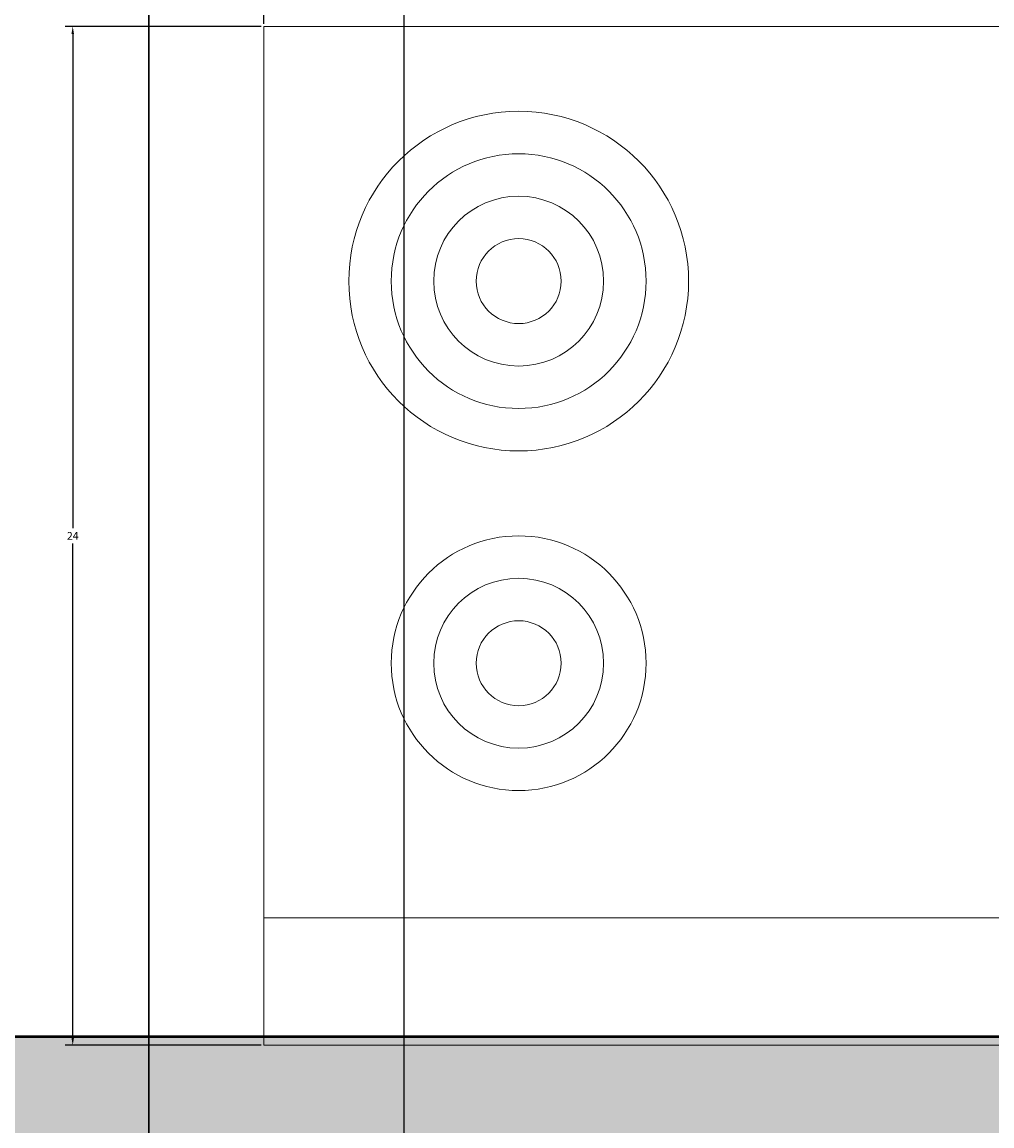
# Model space of a CAD drawing. Units: inches. Extents: x 2307 to 2544, y 2171 to 2540.
# Tile 30 of 52: x 2453 to 2476, y 2317 to 2343. Entities that reach past the tile are written whole.
import ezdxf

# ---------------------------------------------------------------- set-up
doc = ezdxf.new("R2010")
doc.units = ezdxf.units.IN
for name, color, linetype, lineweight in [('A-ANNO-DIMS', 2, 'Continuous', 18), ('A-EQPM', 8, 'Continuous', 18), ('A-WALL', 7, 'Continuous', 50)]:
    doc.layers.add(name, color=color, linetype=linetype, lineweight=lineweight)
doc.layers.add('A-WALL-PATT', color=18, linetype='Continuous', lineweight=13, true_color=0x000000)
doc.styles.get("Standard").update_dxf_attribs({"font": 'arial.ttf'})
doc.dimstyles.get("Standard").update_dxf_attribs({"dimtxt": 0.18, "dimasz": 0.18, "dimexe": 0.18, "dimexo": 0.0625, "dimgap": 0.09, "dimtad": 0, "dimtih": 1, "dimtoh": 1, "dimdec": 4, "dimzin": 0, "dimdsep": 46, "dimtxsty": 'Standard', "dimcen": 0.09, "dimadec": 0, "dimazin": 0, "dimtfac": 1, "dimtdec": 4, "dimtofl": 0, "dimtmove": 0, "dimatfit": 3, "dimfxl": 1, "dimtolj": 1, "dimtzin": 0, "dimarcsym": 0})

# ---------------------------------------------------------------- blocks, each defined once
blk = doc.blocks.new('Range-Oven - 30 in top')
blk.add_line((0, -3), (30, -3))
blk.add_lwpolyline([(0, -24), (0, 0), (30, 0), (30, -24)], close=True)
for centre, radius in [((6, -9), 4), ((6, -9), 3), ((24, -9), 3), ((6, -9), 2), ((24, -9), 2), ((6, -9), 1), ((24, -9), 1), ((24, -18), 4), ((6, -18), 3), ((24, -18), 3), ((6, -18), 2), ((24, -18), 2), ((6, -18), 1), ((24, -18), 1)]:
    blk.add_circle(centre, radius)
blk = doc.blocks.new('*D30')
at = {"layer": 'A-ANNO-DIMS', "color": 0, "lineweight": -2, "transparency": 16777216}
for p, q in [((2458.401, 2343.369), (2458.401, 2347.987)), ((2458.581, 2347.807), (2472.705, 2347.807)), ((2488.221, 2347.807), (2474.097, 2347.807)), ((2488.401, 2343.369), (2488.401, 2347.987))]:
    blk.add_line(p, q, dxfattribs=at)
at = {"layer": 'A-ANNO-DIMS', "color": 0, "transparency": 16777216}
for points in [[(2458.581, 2347.837), (2458.581, 2347.777), (2458.401, 2347.807)], [(2488.221, 2347.837), (2488.221, 2347.777), (2488.401, 2347.807)]]:
    blk.add_solid(points, dxfattribs=at)
at = {"layer": 'Defpoints', "color": 0, "transparency": 16777216}
for p in [(2458.401, 2347.807), (2458.401, 2343.307), (2488.401, 2343.307)]:
    blk.add_point(p, dxfattribs=at)
at = {"layer": 'A-ANNO-DIMS', "color": 0, "transparency": 16777216, "insert": (2473.401, 2347.807), "char_height": 0.18, "attachment_point": 5}
blk.add_mtext('\\A1;RANGE 30', dxfattribs=at)
blk = doc.blocks.new('*D31')
at = {"layer": 'A-ANNO-DIMS', "color": 0, "lineweight": -2, "transparency": 16777216}
for p, q in [((2458.339, 2343.307), (2453.721, 2343.307)), ((2453.901, 2343.127), (2453.901, 2331.487)), ((2453.901, 2319.487), (2453.901, 2331.126)), ((2458.339, 2319.307), (2453.721, 2319.307))]:
    blk.add_line(p, q, dxfattribs=at)
at = {"layer": 'A-ANNO-DIMS', "color": 0, "transparency": 16777216}
for points in [[(2453.871, 2343.127), (2453.931, 2343.127), (2453.901, 2343.307)], [(2453.871, 2319.487), (2453.931, 2319.487), (2453.901, 2319.307)]]:
    blk.add_solid(points, dxfattribs=at)
at = {"layer": 'Defpoints', "color": 0, "transparency": 16777216}
for p in [(2458.401, 2343.307), (2453.901, 2319.307), (2458.401, 2319.307)]:
    blk.add_point(p, dxfattribs=at)
at = {"layer": 'A-ANNO-DIMS', "color": 0, "transparency": 16777216, "insert": (2453.901, 2331.307), "char_height": 0.18, "attachment_point": 5}
blk.add_mtext('\\A1;24', dxfattribs=at)
blk = doc.blocks.new('*D53')
at = {"layer": 'A-ANNO-DIMS', "color": 0, "lineweight": -2, "transparency": 16777216}
for p, q in [((2455.696, 2439.447), (2455.696, 2171.18)), ((2461.696, 2439.447), (2461.696, 2171.18)), ((2455.876, 2171.36), (2458.546, 2171.36)), ((2461.516, 2171.36), (2458.845, 2171.36))]:
    blk.add_line(p, q, dxfattribs=at)
at = {"layer": 'A-ANNO-DIMS', "color": 0, "transparency": 16777216}
for points in [[(2455.876, 2171.39), (2455.876, 2171.33), (2455.696, 2171.36)], [(2461.516, 2171.39), (2461.516, 2171.33), (2461.696, 2171.36)]]:
    blk.add_solid(points, dxfattribs=at)
at = {"layer": 'Defpoints', "color": 0, "transparency": 16777216}
for p in [(2455.696, 2439.51), (2461.696, 2439.51), (2461.696, 2171.36)]:
    blk.add_point(p, dxfattribs=at)
at = {"layer": 'A-ANNO-DIMS', "color": 0, "transparency": 16777216, "insert": (2458.696, 2171.36), "char_height": 0.18, "attachment_point": 5}
blk.add_mtext('\\A1;6', dxfattribs=at)
blk = doc.blocks.new('*D54')
at = {"layer": 'A-ANNO-DIMS', "color": 0, "lineweight": -2, "transparency": 16777216}
for p, q in [((2461.696, 2435.447), (2461.696, 2171.18)), ((2491.696, 2435.447), (2491.696, 2171.18)), ((2461.876, 2171.36), (2476.477, 2171.36)), ((2491.516, 2171.36), (2476.914, 2171.36))]:
    blk.add_line(p, q, dxfattribs=at)
at = {"layer": 'A-ANNO-DIMS', "color": 0, "transparency": 16777216}
for points in [[(2461.876, 2171.39), (2461.876, 2171.33), (2461.696, 2171.36)], [(2491.516, 2171.39), (2491.516, 2171.33), (2491.696, 2171.36)]]:
    blk.add_solid(points, dxfattribs=at)
at = {"layer": 'Defpoints', "color": 0, "transparency": 16777216}
for p in [(2461.696, 2435.51), (2491.696, 2435.51), (2491.696, 2171.36)]:
    blk.add_point(p, dxfattribs=at)
at = {"layer": 'A-ANNO-DIMS', "color": 0, "transparency": 16777216, "insert": (2476.696, 2171.36), "char_height": 0.18, "attachment_point": 5}
blk.add_mtext('\\A1;30', dxfattribs=at)
blk = doc.blocks.new('*D59')
at = {"layer": 'A-ANNO-DIMS', "color": 0, "lineweight": -2, "transparency": 16777216}
for p, q in [((2455.696, 2315.572), (2455.696, 2540.345)), ((2485.696, 2315.572), (2485.696, 2540.345)), ((2455.876, 2540.165), (2470.477, 2540.165)), ((2485.516, 2540.165), (2470.914, 2540.165))]:
    blk.add_line(p, q, dxfattribs=at)
at = {"layer": 'A-ANNO-DIMS', "color": 0, "transparency": 16777216}
for points in [[(2455.876, 2540.195), (2455.876, 2540.135), (2455.696, 2540.165)], [(2485.516, 2540.195), (2485.516, 2540.135), (2485.696, 2540.165)]]:
    blk.add_solid(points, dxfattribs=at)
at = {"layer": 'Defpoints', "color": 0, "transparency": 16777216}
for p in [(2455.696, 2540.165), (2455.696, 2315.51), (2485.696, 2315.51)]:
    blk.add_point(p, dxfattribs=at)
at = {"layer": 'A-ANNO-DIMS', "color": 0, "transparency": 16777216, "insert": (2470.696, 2540.165), "char_height": 0.18, "attachment_point": 5}
blk.add_mtext('\\A1;30', dxfattribs=at)

msp = doc.modelspace()

# ---------------------------------------------------------------- hatches: boundary and pattern name
at = {"layer": 'A-WALL-PATT'}
h = msp.add_hatch(color=256, dxfattribs=at)
h.dxf.hatch_style = 1
h.paths.add_polyline_path([(2433.6935, 2199.5096), (2415.6423, 2199.5096), (2415.6423, 2190.5096), (2433.7832, 2190.5096)], flags=17)
h.paths.add_polyline_path([(2367.6423, 2199.5096), (2335.6958, 2199.5096), (2335.6958, 2307.3983), (2326.6958, 2307.3983), (2326.6958, 2190.5096), (2367.6423, 2190.5096)])
h.paths.add_polyline_path([(2524.6958, 2520.5096), (2496.7832, 2520.5096), (2496.7832, 2515.5149), (2472.7832, 2515.5149), (2472.7832, 2520.5096), (2415.4028, 2520.5096), (2415.4028, 2511.5096), (2451.6958, 2511.5096), (2451.6958, 2439.5096), (2451.6958, 2391.5096), (2445.6958, 2391.5096), (2445.6958, 2387.5096), (2455.6958, 2387.5096), (2455.6958, 2435.5096), (2461.6958, 2435.5096), (2461.6958, 2439.5096), (2455.6958, 2439.5096), (2455.6958, 2511.5096), (2515.6958, 2511.5096), (2515.6958, 2439.5096), (2491.6958, 2439.5096), (2491.6958, 2435.5096), (2515.6958, 2435.5096), (2515.6958, 2319.5096), (2451.6958, 2319.5096), (2451.6958, 2281.5096), (2481.6958, 2281.5096), (2481.6958, 2225.5096), (2485.6958, 2225.5096), (2485.6958, 2285.5096), (2455.6958, 2285.5096), (2455.6958, 2315.5096), (2515.6958, 2315.5096), (2515.6958, 2199.5096), (2469.6952, 2199.5096), (2469.785, 2190.5096), (2524.6958, 2190.5096)])

# ---------------------------------------------------------------- linework, layer by layer
at = {"layer": 'A-WALL'}
msp.add_line((2515.6958, 2319.5096), (2451.6958, 2319.5096), dxfattribs=at)

# ---------------------------------------------------------------- block references
at = {"layer": 'A-EQPM', "rotation": 180}
msp.add_blockref('Range-Oven - 30 in top', (2488.4011, 2319.3068), dxfattribs=at)

# ---------------------------------------------------------------- dimensions: what is measured, and where the dimension line sits
at = {"layer": 'A-ANNO-DIMS'}
for base, p1, p2, picture, middle in [((2455.6958, 2540.1649), (2485.6958, 2315.5096), (2455.6958, 2315.5096), '*D59', (2470.6958, 2540.1649)), ((2461.6958, 2171.3596), (2455.6958, 2439.5096), (2461.6958, 2439.5096), '*D53', (2458.6958, 2171.3596)), ((2491.6958, 2171.3596), (2461.6958, 2435.5096), (2491.6958, 2435.5096), '*D54', (2476.6958, 2171.3596))]:
    dim = msp.add_linear_dim(base=base, p1=p1, p2=p2, dimstyle='Standard', override={"dimdec": 0, "dimlfac": 1, "dimrnd": 0, "dimzin": 0, "dimdsep": 46, "dimlunit": 2}, dxfattribs=at)
    dim.commit()
    dim.dimension.update_dxf_attribs({"geometry": picture, "text_midpoint": middle})
dim = msp.add_linear_dim(base=(2458.4011, 2347.8068), p1=(2488.4011, 2343.3068), p2=(2458.4011, 2343.3068), angle=180, text='RANGE <>', dimstyle='Standard', override={"dimdec": 0, "dimlfac": 1, "dimrnd": 0, "dimzin": 0, "dimdsep": 46, "dimlunit": 2}, dxfattribs=at)
dim.commit()
dim.dimension.update_dxf_attribs({"geometry": '*D30', "text_midpoint": (2473.4011, 2347.8068)})
dim = msp.add_linear_dim(base=(2453.9011, 2319.3068), p1=(2458.4011, 2343.3068), p2=(2458.4011, 2319.3068), angle=270, dimstyle='Standard', override={"dimdec": 0, "dimlfac": 1, "dimrnd": 0, "dimzin": 0, "dimdsep": 46, "dimlunit": 2}, dxfattribs=at)
dim.commit()
dim.dimension.update_dxf_attribs({"geometry": '*D31', "text_midpoint": (2453.9011, 2331.3068)})

doc.saveas('drawing.dxf')
